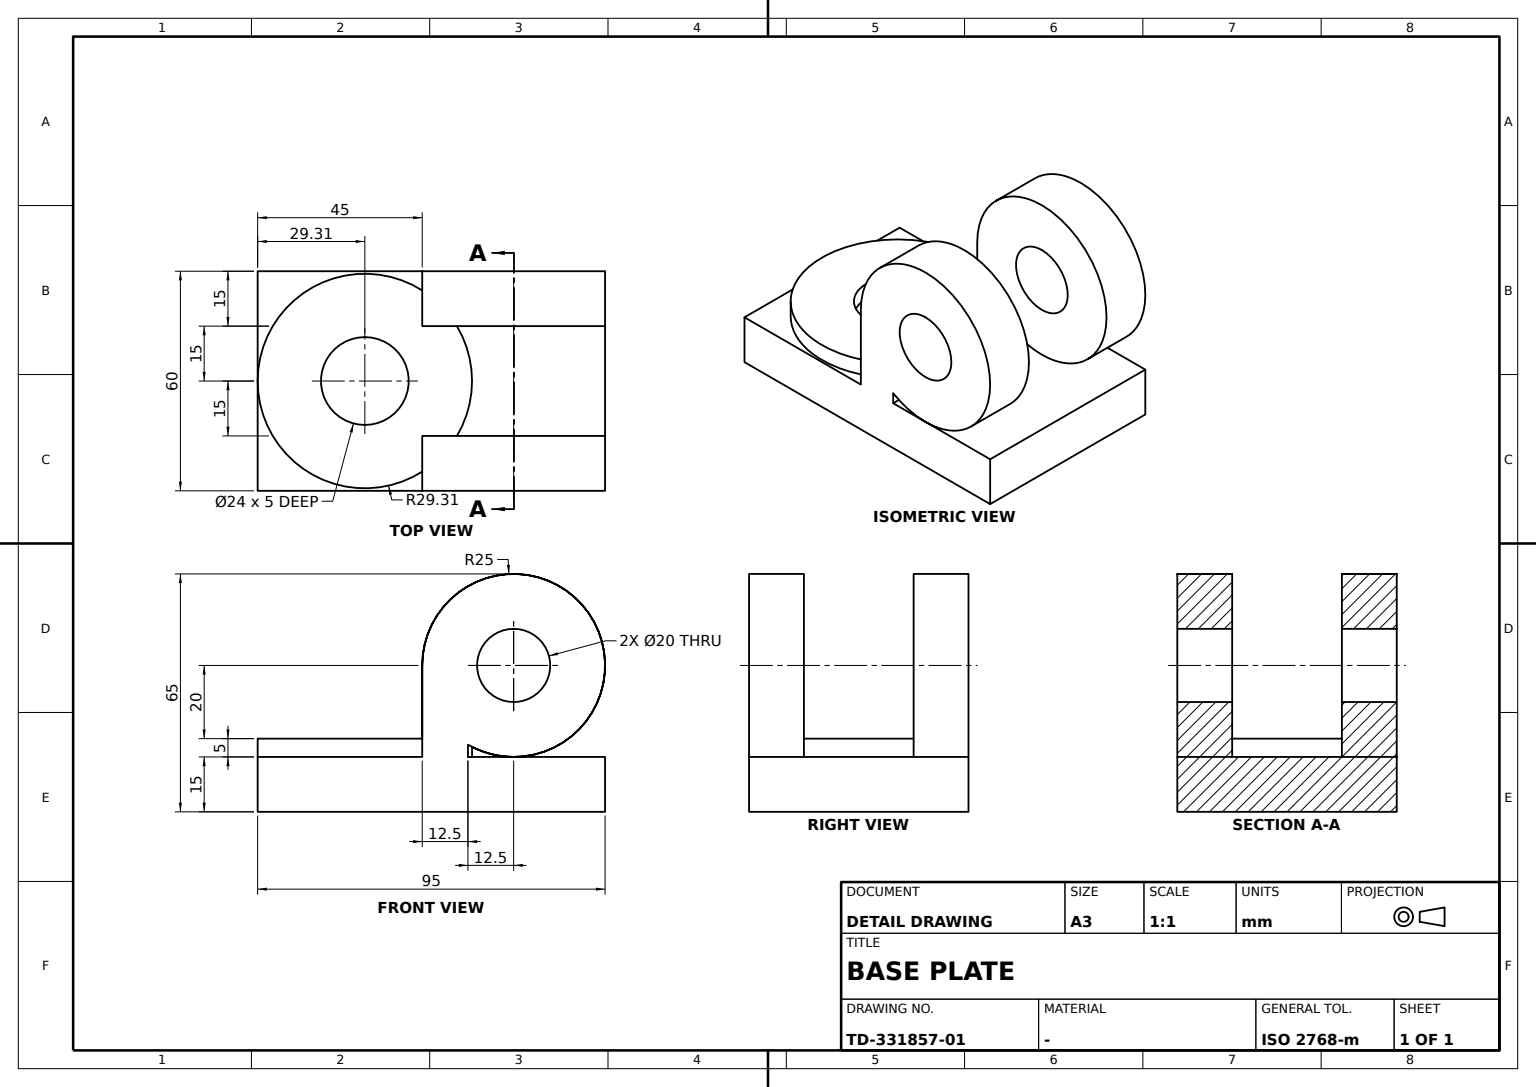
CATIA V5 part; units mm, degrees
sketch "Sketch1" plane through (0, 0, 0) normal (0, 0, 1) x (1, 0, 0)
  line L0 (-30, 47.5) -> (30, 47.5)
  line L1 (30, 47.5) -> (30, -47.5)
  line L2 (30, -47.5) -> (-30, -47.5)
  line L3 (-30, -47.5) -> (-30, 47.5)
  dimension "length L2" = 60
  dimension "length L3" = 95
  constraint horizontal L0 x-axis
  constraint horizontal L2 x-axis
  constraint vertical L1 y-axis
  constraint vertical L3 y-axis
  constraint symmetry L3 L1 y-axis
  constraint symmetry L0 L2 x-axis
extrude "Pad1" add sketch "Sketch1" along normal blind 15
sketch "Sketch2" plane through (0, 0, 15) normal (0, 0, 1) x (1, 0, 0)
  circle A0 centre (0, -18.1897) radius 29.3103
  point P0 (0, -18.1897)
  circle A1 centre (0, -18.1897) radius 12
  line L0 (-30, -47.5) -> (30, -47.5) construction
  dimension "radius A1" = 12
  constraint coincidence P0 y-axis
  constraint tangency L0 A0
extrude "Pad2" add sketch "Sketch2" along normal blind 5
sketch "Sketch3" plane through (-30, 0, 0) normal (-1, 0, 0) x (0, -1, 0)
  point P0 (-47.5, 15)
  point P1 (-47.5, 15)
  arc A0 (2.5, 40) -> (-10, 18.3494) centre (-22.5, 40) ccw
  circle A1 centre (-22.5, 40) radius 10
  line L0 (2.5, 40) -> (2.5, 15)
  line L1 (2.5, 15) -> (-10, 15)
  line L2 (-10, 15) -> (-10, 18.3494)
  dimension "radius A1" = 10
  dimension "radius A0" = 25
  constraint coincidence P0 P1
  constraint tangency L0 A0
  constraint tangency L1 A0
  constraint vertical L2 y-axis
extrude "Pad3" add sketch "Sketch3" against normal blind 15
mirror "Mirror1" about plane through (0, 0, 0) normal (1, 0, 0)
